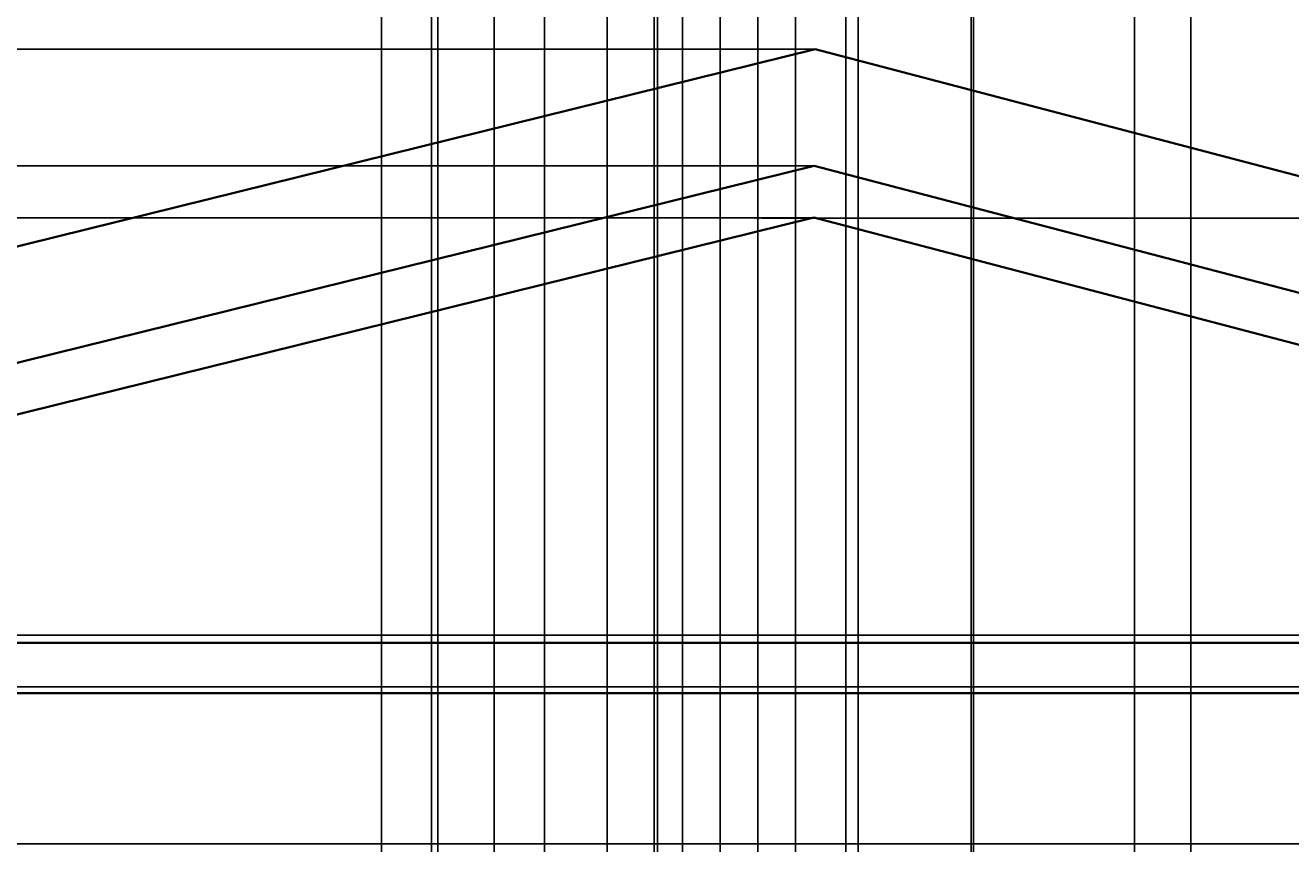
# Model space of a CAD drawing. Units: inches. Extents: x 2154 to 2740, y 571 to 1084.
# Tile 9 of 13: x 2384 to 2485, y 904 to 969. Entities that reach past the tile are written whole.
import ezdxf

# ---------------------------------------------------------------- set-up
doc = ezdxf.new("R2010")
doc.units = ezdxf.units.IN
doc.layers.add('A-ANNO-DIMS', color=2, linetype='Continuous', lineweight=18)
doc.layers.add('A-ROOF', color=1, linetype='Continuous', lineweight=35)
doc.styles.get("Standard").update_dxf_attribs({"font": 'arial.ttf'})
doc.dimstyles.get("Standard").update_dxf_attribs({"dimtxt": 0.18, "dimasz": 0.18, "dimexe": 0.18, "dimexo": 0.0625, "dimgap": 0.09, "dimtad": 0, "dimtih": 1, "dimtoh": 1, "dimdec": 4, "dimzin": 0, "dimdsep": 46, "dimtxsty": 'Standard', "dimcen": 0.09, "dimadec": 0, "dimazin": 0, "dimtfac": 1, "dimtdec": 4, "dimtofl": 0, "dimtmove": 0, "dimatfit": 3, "dimfxl": 1, "dimtolj": 1, "dimtzin": 0, "dimarcsym": 0})

# ---------------------------------------------------------------- blocks, each defined once
blk = doc.blocks.new('*D8')
at = {"layer": 'A-ANNO-DIMS', "color": 0, "lineweight": -2, "transparency": 16777216}
for p, q in [((2284.21, 926.63), (2284.21, 953.59)), ((2284.39, 953.41), (2442.43, 953.37)), ((2601.03, 953.33), (2443, 953.37)), ((2601.21, 926.54), (2601.21, 953.51))]:
    blk.add_line(p, q, dxfattribs=at)
at = {"layer": 'A-ANNO-DIMS', "color": 0, "transparency": 16777216}
for points in [[(2284.39, 953.44), (2284.39, 953.38), (2284.21, 953.41)], [(2601.03, 953.36), (2601.03, 953.3), (2601.21, 953.33)]]:
    blk.add_solid(points, dxfattribs=at)
at = {"layer": 'Defpoints', "color": 0, "transparency": 16777216}
for p in [(2601.21, 953.33), (2284.21, 926.56), (2601.21, 926.48)]:
    blk.add_point(p, dxfattribs=at)
at = {"layer": 'A-ANNO-DIMS', "color": 0, "transparency": 16777216, "insert": (2442.71, 953.37), "char_height": 0.18, "attachment_point": 5}
blk.add_mtext('\\A1;317', dxfattribs=at)
blk = doc.blocks.new('*D9')
at = {"layer": 'A-ANNO-DIMS', "color": 0, "lineweight": -2, "transparency": 16777216}
for p, q in [((2417.21, 970.47), (2417.21, 570.5)), ((2477.21, 970.47), (2477.21, 570.5)), ((2417.39, 570.68), (2446.99, 570.68)), ((2477.03, 570.68), (2447.43, 570.68))]:
    blk.add_line(p, q, dxfattribs=at)
at = {"layer": 'A-ANNO-DIMS', "color": 0, "transparency": 16777216}
for points in [[(2417.39, 570.71), (2417.39, 570.65), (2417.21, 570.68)], [(2477.03, 570.71), (2477.03, 570.65), (2477.21, 570.68)]]:
    blk.add_solid(points, dxfattribs=at)
at = {"layer": 'Defpoints', "color": 0, "transparency": 16777216}
for p in [(2417.21, 970.53), (2477.21, 970.53), (2477.21, 570.68)]:
    blk.add_point(p, dxfattribs=at)
at = {"layer": 'A-ANNO-DIMS', "color": 0, "transparency": 16777216, "insert": (2447.21, 570.68), "char_height": 0.18, "attachment_point": 5}
blk.add_mtext('\\A1;60', dxfattribs=at)
blk = doc.blocks.new('*D10')
at = {"layer": 'A-ANNO-DIMS', "color": 0, "lineweight": -2, "transparency": 16777216}
for p, q in [((2447.14, 1057.01), (2154.18, 1057.01)), ((2154.36, 1056.83), (2154.36, 827.45)), ((2154.36, 597.71), (2154.36, 827.09)), ((2181.14, 597.53), (2154.18, 597.53))]:
    blk.add_line(p, q, dxfattribs=at)
at = {"layer": 'A-ANNO-DIMS', "color": 0, "transparency": 16777216}
for points in [[(2154.33, 1056.83), (2154.39, 1056.83), (2154.36, 1057.01)], [(2154.33, 597.71), (2154.39, 597.71), (2154.36, 597.53)]]:
    blk.add_solid(points, dxfattribs=at)
at = {"layer": 'Defpoints', "color": 0, "transparency": 16777216}
for p in [(2154.36, 1057.01), (2447.21, 1057.01), (2181.21, 597.53)]:
    blk.add_point(p, dxfattribs=at)
at = {"layer": 'A-ANNO-DIMS', "color": 0, "transparency": 16777216, "insert": (2154.36, 827.27), "char_height": 0.18, "attachment_point": 5}
blk.add_mtext('\\A1;459.5', dxfattribs=at)
blk = doc.blocks.new('*D32')
at = {"layer": 'A-ANNO-DIMS', "color": 0, "lineweight": -2, "transparency": 16777216}
for p, q in [((2412.71, 873.59), (2412.71, 1084.04)), ((2412.89, 1083.86), (2442.49, 1083.86)), ((2472.53, 1083.86), (2442.93, 1083.86)), ((2472.71, 873.59), (2472.71, 1084.04))]:
    blk.add_line(p, q, dxfattribs=at)
at = {"layer": 'A-ANNO-DIMS', "color": 0, "transparency": 16777216}
for points in [[(2412.89, 1083.89), (2412.89, 1083.83), (2412.71, 1083.86)], [(2472.53, 1083.89), (2472.53, 1083.83), (2472.71, 1083.86)]]:
    blk.add_solid(points, dxfattribs=at)
at = {"layer": 'Defpoints', "color": 0, "transparency": 16777216}
for p in [(2472.71, 1083.86), (2412.71, 873.53), (2472.71, 873.53)]:
    blk.add_point(p, dxfattribs=at)
at = {"layer": 'A-ANNO-DIMS', "color": 0, "transparency": 16777216, "insert": (2442.71, 1083.86), "char_height": 0.18, "attachment_point": 5}
blk.add_mtext('\\A1;60', dxfattribs=at)
blk = doc.blocks.new('*D35')
at = {"layer": 'A-ANNO-DIMS', "color": 0, "lineweight": -2, "transparency": 16777216}
for p, q in [((2447.21, 966.82), (2154.18, 966.82)), ((2154.36, 966.64), (2154.36, 946.87)), ((2154.36, 926.74), (2154.36, 946.51)), ((2284.14, 926.56), (2154.18, 926.56))]:
    blk.add_line(p, q, dxfattribs=at)
at = {"layer": 'A-ANNO-DIMS', "color": 0, "transparency": 16777216}
for points in [[(2154.33, 966.64), (2154.39, 966.64), (2154.36, 966.82)], [(2154.33, 926.74), (2154.39, 926.74), (2154.36, 926.56)]]:
    blk.add_solid(points, dxfattribs=at)
at = {"layer": 'Defpoints', "color": 0, "transparency": 16777216}
for p in [(2154.36, 966.82), (2447.27, 966.82), (2284.21, 926.56)]:
    blk.add_point(p, dxfattribs=at)
at = {"layer": 'A-ANNO-DIMS', "color": 0, "transparency": 16777216, "insert": (2154.36, 946.69), "char_height": 0.18, "attachment_point": 5}
blk.add_mtext('\\A1;40.255', dxfattribs=at)
blk = doc.blocks.new('*D36')
at = {"layer": 'A-ANNO-DIMS', "color": 0, "lineweight": -2, "transparency": 16777216}
for p, q in [((2447.21, 966.82), (2154.18, 966.82)), ((2154.36, 966.64), (2154.36, 962.36)), ((2154.36, 957.71), (2154.36, 961.99)), ((2447.14, 957.53), (2154.18, 957.53))]:
    blk.add_line(p, q, dxfattribs=at)
at = {"layer": 'A-ANNO-DIMS', "color": 0, "transparency": 16777216}
for points in [[(2154.33, 966.64), (2154.39, 966.64), (2154.36, 966.82)], [(2154.33, 957.71), (2154.39, 957.71), (2154.36, 957.53)]]:
    blk.add_solid(points, dxfattribs=at)
at = {"layer": 'Defpoints', "color": 0, "transparency": 16777216}
for p in [(2154.36, 966.82), (2447.27, 966.82), (2447.21, 957.53)]:
    blk.add_point(p, dxfattribs=at)
at = {"layer": 'A-ANNO-DIMS', "color": 0, "transparency": 16777216, "insert": (2154.36, 962.18), "char_height": 0.18, "attachment_point": 5}
blk.add_mtext('\\A1;9.287', dxfattribs=at)
blk = doc.blocks.new('*D37')
at = {"layer": 'A-ANNO-DIMS', "color": 0, "lineweight": -2, "transparency": 16777216}
for p, q in [((2447.14, 957.53), (2154.18, 957.53)), ((2154.36, 957.35), (2154.36, 955.65)), ((2154.36, 953.58), (2154.36, 955.29)), ((2447.11, 953.4), (2154.18, 953.4))]:
    blk.add_line(p, q, dxfattribs=at)
at = {"layer": 'A-ANNO-DIMS', "color": 0, "transparency": 16777216}
for points in [[(2154.33, 957.35), (2154.39, 957.35), (2154.36, 957.53)], [(2154.33, 953.58), (2154.39, 953.58), (2154.36, 953.4)]]:
    blk.add_solid(points, dxfattribs=at)
at = {"layer": 'Defpoints', "color": 0, "transparency": 16777216}
for p in [(2154.36, 957.53), (2447.21, 957.53), (2447.18, 953.4)]:
    blk.add_point(p, dxfattribs=at)
at = {"layer": 'A-ANNO-DIMS', "color": 0, "transparency": 16777216, "insert": (2154.36, 955.47), "char_height": 0.18, "attachment_point": 5}
blk.add_mtext('\\A1;4.127', dxfattribs=at)
blk = doc.blocks.new('*D38')
at = {"layer": 'A-ANNO-DIMS', "color": 0, "lineweight": -2, "transparency": 16777216}
for p, q in [((2447.11, 953.4), (2154.18, 953.4)), ((2154.36, 953.22), (2154.36, 934.9)), ((2154.36, 916.21), (2154.36, 934.53)), ((2295.71, 916.03), (2154.18, 916.03))]:
    blk.add_line(p, q, dxfattribs=at)
at = {"layer": 'A-ANNO-DIMS', "color": 0, "transparency": 16777216}
for points in [[(2154.33, 953.22), (2154.39, 953.22), (2154.36, 953.4)], [(2154.33, 916.21), (2154.39, 916.21), (2154.36, 916.03)]]:
    blk.add_solid(points, dxfattribs=at)
at = {"layer": 'Defpoints', "color": 0, "transparency": 16777216}
for p in [(2154.36, 953.4), (2447.18, 953.4), (2295.77, 916.03)]:
    blk.add_point(p, dxfattribs=at)
at = {"layer": 'A-ANNO-DIMS', "color": 0, "transparency": 16777216, "insert": (2154.36, 934.72), "char_height": 0.18, "attachment_point": 5}
blk.add_mtext('\\A1;37.38', dxfattribs=at)
blk = doc.blocks.new('*D39')
at = {"layer": 'A-ANNO-DIMS', "color": 0, "lineweight": -2, "transparency": 16777216}
for p, q in [((2183.21, 979.47), (2183.21, 570.5)), ((2417.21, 970.47), (2417.21, 570.5)), ((2183.39, 570.68), (2299.92, 570.68)), ((2417.03, 570.68), (2300.5, 570.68))]:
    blk.add_line(p, q, dxfattribs=at)
at = {"layer": 'A-ANNO-DIMS', "color": 0, "transparency": 16777216}
for points in [[(2183.39, 570.71), (2183.39, 570.65), (2183.21, 570.68)], [(2417.03, 570.71), (2417.03, 570.65), (2417.21, 570.68)]]:
    blk.add_solid(points, dxfattribs=at)
at = {"layer": 'Defpoints', "color": 0, "transparency": 16777216}
for p in [(2183.21, 979.53), (2417.21, 970.53), (2417.21, 570.68)]:
    blk.add_point(p, dxfattribs=at)
at = {"layer": 'A-ANNO-DIMS', "color": 0, "transparency": 16777216, "insert": (2300.21, 570.68), "char_height": 0.18, "attachment_point": 5}
blk.add_mtext('\\A1;234', dxfattribs=at)
blk = doc.blocks.new('*D46')
at = {"layer": 'A-ANNO-DIMS', "color": 0, "lineweight": -2, "transparency": 16777216}
for p, q in [((2195.27, 915.53), (2740.24, 915.53)), ((2740.06, 915.35), (2740.06, 909.71)), ((2740.06, 903.71), (2740.06, 909.35)), ((2195.27, 903.53), (2740.24, 903.53))]:
    blk.add_line(p, q, dxfattribs=at)
at = {"layer": 'A-ANNO-DIMS', "color": 0, "transparency": 16777216}
for points in [[(2740.03, 915.35), (2740.09, 915.35), (2740.06, 915.53)], [(2740.03, 903.71), (2740.09, 903.71), (2740.06, 903.53)]]:
    blk.add_solid(points, dxfattribs=at)
at = {"layer": 'Defpoints', "color": 0, "transparency": 16777216}
for p in [(2195.21, 915.53), (2740.06, 915.53), (2195.21, 903.53)]:
    blk.add_point(p, dxfattribs=at)
at = {"layer": 'A-ANNO-DIMS', "color": 0, "transparency": 16777216, "insert": (2740.06, 909.53), "char_height": 0.18, "attachment_point": 5}
blk.add_mtext('\\A1;12', dxfattribs=at)
blk = doc.blocks.new('*D47')
at = {"layer": 'A-ANNO-DIMS', "color": 0, "lineweight": -2, "transparency": 16777216}
for p, q in [((2195.269199, 919.532069), (2740.236699, 919.532069)), ((2740.056699, 919.352069), (2740.056699, 917.712069)), ((2740.056699, 915.712069), (2740.056699, 917.352069)), ((2195.269199, 915.532069), (2740.236699, 915.532069))]:
    blk.add_line(p, q, dxfattribs=at)
at = {"layer": 'A-ANNO-DIMS', "color": 0, "transparency": 16777216}
for points in [[(2740.026699, 919.352069), (2740.086699, 919.352069), (2740.056699, 919.532069)], [(2740.026699, 915.712069), (2740.086699, 915.712069), (2740.056699, 915.532069)]]:
    blk.add_solid(points, dxfattribs=at)
at = {"layer": 'Defpoints', "color": 0, "transparency": 16777216}
for p in [(2195.206699, 919.532069), (2740.056699, 919.532069), (2195.206699, 915.532069)]:
    blk.add_point(p, dxfattribs=at)
at = {"layer": 'A-ANNO-DIMS', "color": 0, "transparency": 16777216, "insert": (2740.056699, 917.532069), "char_height": 0.18, "attachment_point": 5}
blk.add_mtext('\\A1;4', dxfattribs=at)
blk = doc.blocks.new('*D48')
at = {"layer": 'A-ANNO-DIMS', "color": 0, "lineweight": -2, "transparency": 16777216}
for p, q in [((2195.27, 979.53), (2740.24, 979.53)), ((2740.06, 979.35), (2740.06, 949.71)), ((2740.06, 919.71), (2740.06, 949.35)), ((2195.27, 919.53), (2740.24, 919.53))]:
    blk.add_line(p, q, dxfattribs=at)
at = {"layer": 'A-ANNO-DIMS', "color": 0, "transparency": 16777216}
for points in [[(2740.03, 979.35), (2740.09, 979.35), (2740.06, 979.53)], [(2740.03, 919.71), (2740.09, 919.71), (2740.06, 919.53)]]:
    blk.add_solid(points, dxfattribs=at)
at = {"layer": 'Defpoints', "color": 0, "transparency": 16777216}
for p in [(2195.21, 979.53), (2740.06, 979.53), (2195.21, 919.53)]:
    blk.add_point(p, dxfattribs=at)
at = {"layer": 'A-ANNO-DIMS', "color": 0, "transparency": 16777216, "insert": (2740.06, 949.53), "char_height": 0.18, "attachment_point": 5}
blk.add_mtext('\\A1;60', dxfattribs=at)
blk = doc.blocks.new('*D55')
at = {"layer": 'A-ANNO-DIMS', "color": 0, "lineweight": -2, "transparency": 16777216}
for p, q in [((2295.84, 920.15), (2740.24, 920.15)), ((2740.06, 919.97), (2740.06, 918.27)), ((2740.06, 916.21), (2740.06, 917.91)), ((2295.83, 916.03), (2740.24, 916.03))]:
    blk.add_line(p, q, dxfattribs=at)
at = {"layer": 'A-ANNO-DIMS', "color": 0, "transparency": 16777216}
for points in [[(2740.03, 919.97), (2740.09, 919.97), (2740.06, 920.15)], [(2740.03, 916.21), (2740.09, 916.21), (2740.06, 916.03)]]:
    blk.add_solid(points, dxfattribs=at)
at = {"layer": 'Defpoints', "color": 0, "transparency": 16777216}
for p in [(2295.77, 920.15), (2740.06, 920.15), (2295.77, 916.03)]:
    blk.add_point(p, dxfattribs=at)
at = {"layer": 'A-ANNO-DIMS', "color": 0, "transparency": 16777216, "insert": (2740.06, 918.09), "char_height": 0.18, "attachment_point": 5}
blk.add_mtext('\\A1;4.12', dxfattribs=at)
blk = doc.blocks.new('*D75')
at = {"layer": 'A-ANNO-DIMS', "color": 0, "lineweight": -2, "transparency": 16777216}
for p, q in [((2434.46, 990.57), (2434.46, 570.5)), ((2417.21, 981.47), (2417.21, 570.5)), ((2417.39, 570.68), (2425.45, 570.68)), ((2434.28, 570.68), (2426.22, 570.68))]:
    blk.add_line(p, q, dxfattribs=at)
at = {"layer": 'A-ANNO-DIMS', "color": 0, "transparency": 16777216}
for points in [[(2417.39, 570.71), (2417.39, 570.65), (2417.21, 570.68)], [(2434.28, 570.71), (2434.28, 570.65), (2434.46, 570.68)]]:
    blk.add_solid(points, dxfattribs=at)
at = {"layer": 'Defpoints', "color": 0, "transparency": 16777216}
for p in [(2434.46, 990.64), (2417.21, 981.53), (2434.46, 570.68)]:
    blk.add_point(p, dxfattribs=at)
at = {"layer": 'A-ANNO-DIMS', "color": 0, "transparency": 16777216, "insert": (2425.83, 570.68), "char_height": 0.18, "attachment_point": 5}
blk.add_mtext('\\A1;17.25', dxfattribs=at)
blk = doc.blocks.new('*D76')
at = {"layer": 'A-ANNO-DIMS', "color": 0, "lineweight": -2, "transparency": 16777216}
for p, q in [((2434.46, 990.57), (2434.46, 570.5)), ((2459.89, 990.57), (2459.89, 570.5)), ((2434.64, 570.68), (2446.71, 570.68)), ((2459.71, 570.68), (2447.64, 570.68))]:
    blk.add_line(p, q, dxfattribs=at)
at = {"layer": 'A-ANNO-DIMS', "color": 0, "transparency": 16777216}
for points in [[(2434.64, 570.71), (2434.64, 570.65), (2434.46, 570.68)], [(2459.71, 570.71), (2459.71, 570.65), (2459.89, 570.68)]]:
    blk.add_solid(points, dxfattribs=at)
at = {"layer": 'Defpoints', "color": 0, "transparency": 16777216}
for p in [(2434.46, 990.64), (2459.89, 990.64), (2459.89, 570.68)]:
    blk.add_point(p, dxfattribs=at)
at = {"layer": 'A-ANNO-DIMS', "color": 0, "transparency": 16777216, "insert": (2447.17, 570.68), "char_height": 0.18, "attachment_point": 5}
blk.add_mtext('\\A1;25.433', dxfattribs=at)
blk = doc.blocks.new('*D87')
at = {"layer": 'A-ANNO-DIMS', "color": 0, "lineweight": -2, "transparency": 16777216}
for p, q in [((2421.71, 725.29), (2421.71, 1084.04)), ((2421.89, 1083.86), (2423.55, 1083.86)), ((2425.53, 1083.86), (2423.86, 1083.86)), ((2425.71, 721.29), (2425.71, 1084.04))]:
    blk.add_line(p, q, dxfattribs=at)
at = {"layer": 'A-ANNO-DIMS', "color": 0, "transparency": 16777216}
for points in [[(2421.89, 1083.89), (2421.89, 1083.83), (2421.71, 1083.86)], [(2425.53, 1083.89), (2425.53, 1083.83), (2425.71, 1083.86)]]:
    blk.add_solid(points, dxfattribs=at)
at = {"layer": 'Defpoints', "color": 0, "transparency": 16777216}
for p in [(2425.71, 1083.86), (2421.71, 725.23), (2425.71, 721.23)]:
    blk.add_point(p, dxfattribs=at)
at = {"layer": 'A-ANNO-DIMS', "color": 0, "transparency": 16777216, "insert": (2423.71, 1083.86), "char_height": 0.18, "attachment_point": 5}
blk.add_mtext('\\A1;4', dxfattribs=at)
blk = doc.blocks.new('*D90')
at = {"layer": 'A-ANNO-DIMS', "color": 0, "lineweight": -2, "transparency": 16777216}
for p, q in [((2434.71, 712.29), (2434.71, 1084.04)), ((2434.89, 1083.86), (2442.5, 1083.86)), ((2450.53, 1083.86), (2442.92, 1083.86)), ((2450.71, 712.29), (2450.71, 1084.04))]:
    blk.add_line(p, q, dxfattribs=at)
at = {"layer": 'A-ANNO-DIMS', "color": 0, "transparency": 16777216}
for points in [[(2434.89, 1083.89), (2434.89, 1083.83), (2434.71, 1083.86)], [(2450.53, 1083.89), (2450.53, 1083.83), (2450.71, 1083.86)]]:
    blk.add_solid(points, dxfattribs=at)
at = {"layer": 'Defpoints', "color": 0, "transparency": 16777216}
for p in [(2450.71, 1083.86), (2434.71, 712.23), (2450.71, 712.23)]:
    blk.add_point(p, dxfattribs=at)
at = {"layer": 'A-ANNO-DIMS', "color": 0, "transparency": 16777216, "insert": (2442.71, 1083.86), "char_height": 0.18, "attachment_point": 5}
blk.add_mtext('\\A1;16', dxfattribs=at)
blk = doc.blocks.new('*D93')
at = {"layer": 'A-ANNO-DIMS', "color": 0, "lineweight": -2, "transparency": 16777216}
for p, q in [((2439.71, 703.29), (2439.71, 1084.04)), ((2439.89, 1083.86), (2442.56, 1083.86)), ((2445.53, 1083.86), (2442.86, 1083.86)), ((2445.71, 703.29), (2445.71, 1084.04))]:
    blk.add_line(p, q, dxfattribs=at)
at = {"layer": 'A-ANNO-DIMS', "color": 0, "transparency": 16777216}
for points in [[(2439.89, 1083.89), (2439.89, 1083.83), (2439.71, 1083.86)], [(2445.53, 1083.89), (2445.53, 1083.83), (2445.71, 1083.86)]]:
    blk.add_solid(points, dxfattribs=at)
at = {"layer": 'Defpoints', "color": 0, "transparency": 16777216}
for p in [(2445.71, 1083.86), (2439.71, 703.23), (2445.71, 703.23)]:
    blk.add_point(p, dxfattribs=at)
at = {"layer": 'A-ANNO-DIMS', "color": 0, "transparency": 16777216, "insert": (2442.71, 1083.86), "char_height": 0.18, "attachment_point": 5}
blk.add_mtext('\\A1;6', dxfattribs=at)
blk = doc.blocks.new('*D94')
at = {"layer": 'A-ANNO-DIMS', "color": 0, "lineweight": -2, "transparency": 16777216}
for p, q in [((2445.71, 703.29), (2445.71, 1084.04)), ((2445.89, 1083.86), (2447.55, 1083.86)), ((2449.53, 1083.86), (2447.86, 1083.86)), ((2449.71, 703.29), (2449.71, 1084.04))]:
    blk.add_line(p, q, dxfattribs=at)
at = {"layer": 'A-ANNO-DIMS', "color": 0, "transparency": 16777216}
for points in [[(2445.89, 1083.89), (2445.89, 1083.83), (2445.71, 1083.86)], [(2449.53, 1083.89), (2449.53, 1083.83), (2449.71, 1083.86)]]:
    blk.add_solid(points, dxfattribs=at)
at = {"layer": 'Defpoints', "color": 0, "transparency": 16777216}
for p in [(2449.71, 1083.86), (2445.71, 703.23), (2449.71, 703.23)]:
    blk.add_point(p, dxfattribs=at)
at = {"layer": 'A-ANNO-DIMS', "color": 0, "transparency": 16777216, "insert": (2447.71, 1083.86), "char_height": 0.18, "attachment_point": 5}
blk.add_mtext('\\A1;4', dxfattribs=at)
blk = doc.blocks.new('*D99')
at = {"layer": 'A-ANNO-DIMS', "color": 0, "lineweight": -2, "transparency": 16777216}
for p, q in [((2412.71, 873.59), (2412.71, 1084.04)), ((2412.89, 1083.86), (2414.55, 1083.86)), ((2416.53, 1083.86), (2414.86, 1083.86)), ((2416.71, 869.59), (2416.71, 1084.04))]:
    blk.add_line(p, q, dxfattribs=at)
at = {"layer": 'A-ANNO-DIMS', "color": 0, "transparency": 16777216}
for points in [[(2412.89, 1083.89), (2412.89, 1083.83), (2412.71, 1083.86)], [(2416.53, 1083.89), (2416.53, 1083.83), (2416.71, 1083.86)]]:
    blk.add_solid(points, dxfattribs=at)
at = {"layer": 'Defpoints', "color": 0, "transparency": 16777216}
for p in [(2416.71, 1083.86), (2412.71, 873.53), (2416.71, 869.53)]:
    blk.add_point(p, dxfattribs=at)
at = {"layer": 'A-ANNO-DIMS', "color": 0, "transparency": 16777216, "insert": (2414.71, 1083.86), "char_height": 0.18, "attachment_point": 5}
blk.add_mtext('\\A1;4', dxfattribs=at)
blk = doc.blocks.new('*D101')
at = {"layer": 'A-ANNO-DIMS', "color": 0, "lineweight": -2, "transparency": 16777216}
for p, q in [((2416.71, 869.59), (2416.71, 1084.04)), ((2416.89, 1083.86), (2421.06, 1083.86)), ((2425.53, 1083.86), (2421.36, 1083.86)), ((2425.71, 860.59), (2425.71, 1084.04))]:
    blk.add_line(p, q, dxfattribs=at)
at = {"layer": 'A-ANNO-DIMS', "color": 0, "transparency": 16777216}
for points in [[(2416.89, 1083.89), (2416.89, 1083.83), (2416.71, 1083.86)], [(2425.53, 1083.89), (2425.53, 1083.83), (2425.71, 1083.86)]]:
    blk.add_solid(points, dxfattribs=at)
at = {"layer": 'Defpoints', "color": 0, "transparency": 16777216}
for p in [(2425.71, 1083.86), (2416.71, 869.53), (2425.71, 860.53)]:
    blk.add_point(p, dxfattribs=at)
at = {"layer": 'A-ANNO-DIMS', "color": 0, "transparency": 16777216, "insert": (2421.21, 1083.86), "char_height": 0.18, "attachment_point": 5}
blk.add_mtext('\\A1;9', dxfattribs=at)
blk = doc.blocks.new('*D102')
at = {"layer": 'A-ANNO-DIMS', "color": 0, "lineweight": -2, "transparency": 16777216}
for p, q in [((2425.71, 860.59), (2425.71, 1084.04)), ((2425.89, 1083.86), (2428.06, 1083.86)), ((2430.53, 1083.86), (2428.36, 1083.86)), ((2430.71, 860.59), (2430.71, 1084.04))]:
    blk.add_line(p, q, dxfattribs=at)
at = {"layer": 'A-ANNO-DIMS', "color": 0, "transparency": 16777216}
for points in [[(2425.89, 1083.89), (2425.89, 1083.83), (2425.71, 1083.86)], [(2430.53, 1083.89), (2430.53, 1083.83), (2430.71, 1083.86)]]:
    blk.add_solid(points, dxfattribs=at)
at = {"layer": 'Defpoints', "color": 0, "transparency": 16777216}
for p in [(2430.71, 1083.86), (2425.71, 860.53), (2430.71, 860.53)]:
    blk.add_point(p, dxfattribs=at)
at = {"layer": 'A-ANNO-DIMS', "color": 0, "transparency": 16777216, "insert": (2428.21, 1083.86), "char_height": 0.18, "attachment_point": 5}
blk.add_mtext('\\A1;5', dxfattribs=at)
blk = doc.blocks.new('*D103')
at = {"layer": 'A-ANNO-DIMS', "color": 0, "lineweight": -2, "transparency": 16777216}
for p, q in [((2430.71, 860.59), (2430.71, 1084.04)), ((2430.89, 1083.86), (2433.56, 1083.86)), ((2436.53, 1083.86), (2433.86, 1083.86)), ((2436.71, 860.59), (2436.71, 1084.04))]:
    blk.add_line(p, q, dxfattribs=at)
at = {"layer": 'A-ANNO-DIMS', "color": 0, "transparency": 16777216}
for points in [[(2430.89, 1083.89), (2430.89, 1083.83), (2430.71, 1083.86)], [(2436.53, 1083.89), (2436.53, 1083.83), (2436.71, 1083.86)]]:
    blk.add_solid(points, dxfattribs=at)
at = {"layer": 'Defpoints', "color": 0, "transparency": 16777216}
for p in [(2436.71, 1083.86), (2430.71, 860.53), (2436.71, 860.53)]:
    blk.add_point(p, dxfattribs=at)
at = {"layer": 'A-ANNO-DIMS', "color": 0, "transparency": 16777216, "insert": (2433.71, 1083.86), "char_height": 0.18, "attachment_point": 5}
blk.add_mtext('\\A1;6', dxfattribs=at)
blk = doc.blocks.new('*D104')
at = {"layer": 'A-ANNO-DIMS', "color": 0, "lineweight": -2, "transparency": 16777216}
for p, q in [((2436.71, 860.59), (2436.71, 1084.04)), ((2436.89, 1083.86), (2439.56, 1083.86)), ((2442.53, 1083.86), (2439.86, 1083.86)), ((2442.71, 860.59), (2442.71, 1084.04))]:
    blk.add_line(p, q, dxfattribs=at)
at = {"layer": 'A-ANNO-DIMS', "color": 0, "transparency": 16777216}
for points in [[(2436.89, 1083.89), (2436.89, 1083.83), (2436.71, 1083.86)], [(2442.53, 1083.89), (2442.53, 1083.83), (2442.71, 1083.86)]]:
    blk.add_solid(points, dxfattribs=at)
at = {"layer": 'Defpoints', "color": 0, "transparency": 16777216}
for p in [(2442.71, 1083.86), (2436.71, 860.53), (2442.71, 860.53)]:
    blk.add_point(p, dxfattribs=at)
at = {"layer": 'A-ANNO-DIMS', "color": 0, "transparency": 16777216, "insert": (2439.71, 1083.86), "char_height": 0.18, "attachment_point": 5}
blk.add_mtext('\\A1;6', dxfattribs=at)
blk = doc.blocks.new('*D105')
at = {"layer": 'A-ANNO-DIMS', "color": 0, "lineweight": -2, "transparency": 16777216}
for p, q in [((2442.71, 860.59), (2442.71, 1084.04)), ((2442.89, 1083.86), (2451, 1083.86)), ((2459.53, 1083.86), (2451.42, 1083.86)), ((2459.71, 860.59), (2459.71, 1084.04))]:
    blk.add_line(p, q, dxfattribs=at)
at = {"layer": 'A-ANNO-DIMS', "color": 0, "transparency": 16777216}
for points in [[(2442.89, 1083.89), (2442.89, 1083.83), (2442.71, 1083.86)], [(2459.53, 1083.89), (2459.53, 1083.83), (2459.71, 1083.86)]]:
    blk.add_solid(points, dxfattribs=at)
at = {"layer": 'Defpoints', "color": 0, "transparency": 16777216}
for p in [(2459.71, 1083.86), (2442.71, 860.53), (2459.71, 860.53)]:
    blk.add_point(p, dxfattribs=at)
at = {"layer": 'A-ANNO-DIMS', "color": 0, "transparency": 16777216, "insert": (2451.21, 1083.86), "char_height": 0.18, "attachment_point": 5}
blk.add_mtext('\\A1;17', dxfattribs=at)

msp = doc.modelspace()

# ---------------------------------------------------------------- linework, layer by layer
at = {"layer": 'A-ROOF'}
for p, q in [((2447.273, 966.8186), (2284.2067, 926.5633)), ((2447.273, 966.8186), (2601.2067, 926.4774)), ((2447.2067, 957.5321), (2295.7731, 920.1485)), ((2447.2067, 957.5321), (2590.2325, 920.0494)), ((2447.1772, 953.4047), (2295.7714, 916.028)), ((2447.1772, 953.4047), (2590.1732, 915.9299)), ((2309.9659, 919.5321), (2576.4281, 919.5321)), ((2195.2067, 915.5321), (2699.2067, 915.5321))]:
    msp.add_line(p, q, dxfattribs=at)

# ---------------------------------------------------------------- dimensions: what is measured, and where the dimension line sits
at = {"layer": 'A-ANNO-DIMS'}
for base, p1, p2, override, picture, middle in [((2472.7067, 1083.8553), (2412.7067, 873.5321), (2472.7067, 873.5321), {"dimdec": 0, "dimlfac": 1, "dimrnd": 0, "dimzin": 0, "dimdsep": 46, "dimlunit": 2}, '*D32', (2442.7067, 1083.8553)), ((2416.7067, 1083.8553), (2412.7067, 873.5321), (2416.7067, 869.5321), {"dimdec": 0, "dimlfac": 1, "dimrnd": 0, "dimzin": 0, "dimdsep": 46, "dimlunit": 2}, '*D99', (2414.7067, 1083.8553)), ((2425.7067, 1083.8553), (2416.7067, 869.5321), (2425.7067, 860.5321), {"dimdec": 0, "dimlfac": 1, "dimrnd": 0, "dimzin": 0, "dimdsep": 46, "dimlunit": 2}, '*D101', (2421.2067, 1083.8553)), ((2425.7067, 1083.8553), (2421.7067, 725.2281), (2425.7067, 721.2281), {"dimdec": 0, "dimlfac": 1, "dimrnd": 0, "dimzin": 0, "dimdsep": 46, "dimlunit": 2}, '*D87', (2423.7067, 1083.8553)), ((2430.7067, 1083.8553), (2425.7067, 860.5321), (2430.7067, 860.5321), {"dimdec": 0, "dimlfac": 1, "dimrnd": 0, "dimzin": 0, "dimdsep": 46, "dimlunit": 2}, '*D102', (2428.2067, 1083.8553)), ((2436.7067, 1083.8553), (2430.7067, 860.5321), (2436.7067, 860.5321), {"dimdec": 0, "dimlfac": 1, "dimrnd": 0, "dimzin": 0, "dimdsep": 46, "dimlunit": 2}, '*D103', (2433.7067, 1083.8553)), ((2450.7067, 1083.8553), (2434.7067, 712.2281), (2450.7067, 712.2281), {"dimdec": 0, "dimlfac": 1, "dimrnd": 0, "dimzin": 0, "dimdsep": 46, "dimlunit": 2}, '*D90', (2442.7067, 1083.8553)), ((2442.7067, 1083.8553), (2436.7067, 860.5321), (2442.7067, 860.5321), {"dimdec": 0, "dimlfac": 1, "dimrnd": 0, "dimzin": 0, "dimdsep": 46, "dimlunit": 2}, '*D104', (2439.7067, 1083.8553)), ((2445.7067, 1083.8553), (2439.7067, 703.2281), (2445.7067, 703.2281), {"dimdec": 0, "dimlfac": 1, "dimrnd": 0, "dimzin": 0, "dimdsep": 46, "dimlunit": 2}, '*D93', (2442.7067, 1083.8553)), ((2459.7067, 1083.8553), (2442.7067, 860.5321), (2459.7067, 860.5321), {"dimdec": 0, "dimlfac": 1, "dimrnd": 0, "dimzin": 0, "dimdsep": 46, "dimlunit": 2}, '*D105', (2451.2067, 1083.8553)), ((2449.7067, 1083.8553), (2445.7067, 703.2281), (2449.7067, 703.2281), {"dimdec": 0, "dimlfac": 1, "dimrnd": 0, "dimzin": 0, "dimdsep": 46, "dimlunit": 2}, '*D94', (2447.7067, 1083.8553)), ((2434.4565, 570.6821), (2417.2067, 981.5321), (2434.4565, 990.6361), {"dimdec": 2, "dimlfac": 1, "dimrnd": 0, "dimzin": 0, "dimdsep": 46, "dimlunit": 2}, '*D75', (2425.8316, 570.6821)), ((2459.8896, 570.6821), (2434.4565, 990.6361), (2459.8896, 990.6361), {"dimdec": 3, "dimlfac": 1, "dimrnd": 0, "dimzin": 0, "dimdsep": 46, "dimlunit": 2}, '*D76', (2447.173, 570.6821)), ((2417.2067, 570.6821), (2183.2067, 979.5321), (2417.2067, 970.5321), {"dimdec": 0, "dimlfac": 1, "dimrnd": 0, "dimzin": 0, "dimdsep": 46, "dimlunit": 2}, '*D39', (2300.2067, 570.6821)), ((2477.2067, 570.6821), (2417.2067, 970.5321), (2477.2067, 970.5321), {"dimdec": 0, "dimlfac": 1, "dimrnd": 0, "dimzin": 0, "dimdsep": 46, "dimlunit": 2}, '*D9', (2447.2067, 570.6821))]:
    dim = msp.add_linear_dim(base=base, p1=p1, p2=p2, dimstyle='Standard', override=override, dxfattribs=at)
    dim.commit()
    dim.dimension.update_dxf_attribs({"geometry": picture, "text_midpoint": middle})
for base, p1, p2, angle, override, picture, middle in [((2154.3567, 1057.0053), (2181.2067, 597.5321), (2447.2067, 1057.0053), 90, {"dimdec": 1, "dimlfac": 1, "dimrnd": 0, "dimzin": 0, "dimdsep": 46, "dimlunit": 2}, '*D10', (2154.3567, 827.2687)), ((2740.0567, 979.5321), (2195.2067, 919.5321), (2195.2067, 979.5321), 90, {"dimdec": 0, "dimlfac": 1, "dimrnd": 0, "dimzin": 0, "dimdsep": 46, "dimlunit": 2}, '*D48', (2740.0567, 949.5321)), ((2154.3567, 966.8186), (2284.2067, 926.5633), (2447.273, 966.8186), 90, {"dimdec": 3, "dimlfac": 1, "dimrnd": 0, "dimzin": 0, "dimdsep": 46, "dimlunit": 2}, '*D35', (2154.3567, 946.691)), ((2154.3567, 966.81862), (2447.2067, 957.53207), (2447.273, 966.81862), 90, {"dimdec": 3, "dimlfac": 1, "dimrnd": 0, "dimzin": 0, "dimdsep": 46, "dimlunit": 2}, '*D36', (2154.3567, 962.17534)), ((2154.3567, 957.5321), (2447.1772, 953.4047), (2447.2067, 957.5321), 90, {"dimdec": 3, "dimlfac": 1, "dimrnd": 0, "dimzin": 0, "dimdsep": 46, "dimlunit": 2}, '*D37', (2154.3567, 955.4684)), ((2154.3567, 953.4047), (2295.7714, 916.028), (2447.1772, 953.4047), 90, {"dimdec": 2, "dimlfac": 1, "dimrnd": 0, "dimzin": 0, "dimdsep": 46, "dimlunit": 2}, '*D38', (2154.3567, 934.7163)), ((2601.214, 953.3274), (2284.2067, 926.5633), (2601.2067, 926.4774), 359.984471, {"dimdec": 0, "dimlfac": 1, "dimrnd": 0, "dimzin": 0, "dimdsep": 46, "dimlunit": 2}, '*D8', (2442.714, 953.3703)), ((2740.0567, 919.5321), (2195.2067, 915.5321), (2195.2067, 919.5321), 90, {"dimdec": 0, "dimlfac": 1, "dimrnd": 0, "dimzin": 0, "dimdsep": 46, "dimlunit": 2}, '*D47', (2740.0567, 917.5321)), ((2740.0567, 920.1485), (2295.7714, 916.028), (2295.7731, 920.1485), 90, {"dimdec": 2, "dimlfac": 1, "dimrnd": 0, "dimzin": 0, "dimdsep": 46, "dimlunit": 2}, '*D55', (2740.0567, 918.0882)), ((2740.0567, 915.5321), (2195.2067, 903.5321), (2195.2067, 915.5321), 90, {"dimdec": 0, "dimlfac": 1, "dimrnd": 0, "dimzin": 0, "dimdsep": 46, "dimlunit": 2}, '*D46', (2740.0567, 909.5321))]:
    dim = msp.add_linear_dim(base=base, p1=p1, p2=p2, angle=angle, dimstyle='Standard', override=override, dxfattribs=at)
    dim.commit()
    dim.dimension.update_dxf_attribs({"geometry": picture, "text_midpoint": middle})

doc.saveas('drawing.dxf')
